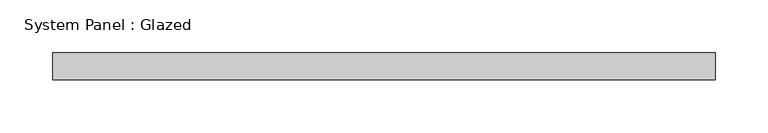
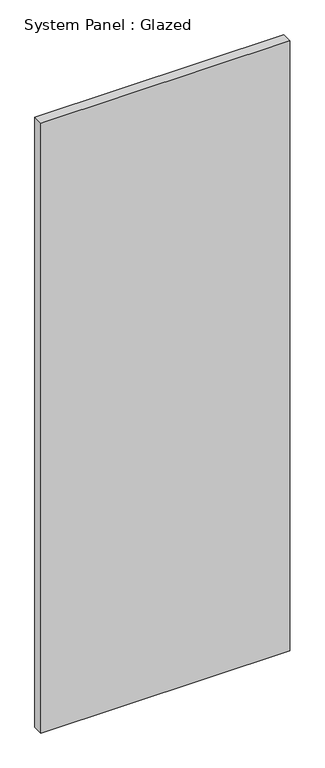
"""IFC4 building model written with IfcOpenShell, lengths in millimetres: plate geometry, System Panel : Glazed."""

from ifc_helpers import new_model, si_unit, origin, origin_with_axes, place, context, project, spatial, polyline, outline, extrude, source, transform, mapped, element, save


def system_panel_glazed_404d015f(model_context):
    return source(origin(), model_context, "Body", "SweptSolid", [
        extrude(outline(polyline([(313.8552609, 19.05), (-313.8552609, 19.05), (-313.8552609, 44.45), (313.8552609, 44.45), (313.8552609, 19.05)])), origin_with_axes(), (0.0, 0.0, 1.0), 1625.6),
    ])


if __name__ == "__main__":
    model = new_model("IFC4")
    model_context = context("Model", 3, world=origin())
    ifc_project = project(units=[si_unit("LENGTHUNIT", "METRE", prefix="MILLI")], contexts=[model_context])
    site = spatial("IfcSite", under=ifc_project)
    building = spatial("IfcBuilding", under=site)
    placement = place(None, origin())
    system_panel_glazed_shape = system_panel_glazed_404d015f(model_context)
    element("IfcPlate", 1, ObjectType="System Panel : Glazed", at=placement, inside=building, context=model_context, shape_type="MappedRepresentation", body=[
        mapped(system_panel_glazed_shape, transform((0.0, 0.0, 0.0), x_axis=(1.0, 0.0, 0.0), y_axis=(0.0, 1.0, 0.0), z_axis=(0.0, 0.0, 1.0))),
    ])
    save(model, "model.ifc")

# Revit data of these elements
# Type "System Panel : Glazed"
#   Construction Type Id = "GSP4R"
#   Analytic Construction = "1/8 in Pilkington single glazing"
#   Visual Light Transmittance = 0.9
#   Solar Heat Gain Coefficient = 0.86
#   Heat Transfer Coefficient (U) = 1.18115 BTU/(h·ft²·°F)
# Element 1 (IfcPlate, "System Panel : Glazed")
#   Materials on its faces: "Glass"
# Materials
#   "Glass": class "Glass", colour RGB 0 128 192, transparency 0.75, Description = "Soda Lime Glass", Cost = 0
